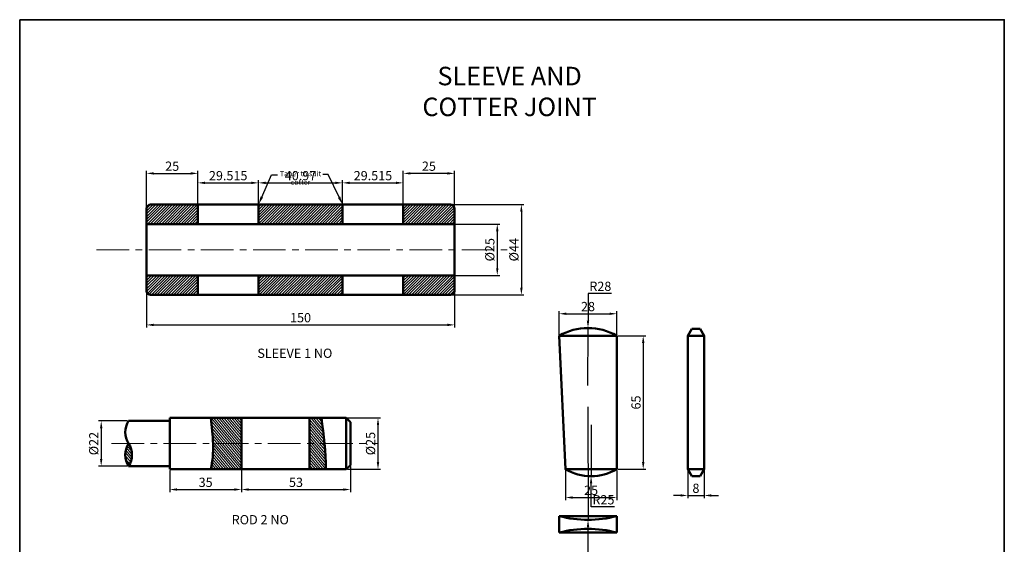
# Model space of a CAD drawing. Units: millimetres. Extents: x -431 to 49, y 153 to 670.
# Tile 2 of 2: x -431 to 49, y 415 to 670. Entities that reach past the tile are written whole.
import ezdxf
from ezdxf import colors
from ezdxf.entities.mleader import LeaderData, LeaderLine
from ezdxf.math import Vec2, Vec3

# ---------------------------------------------------------------- set-up
doc = ezdxf.new("R2010")
doc.units = ezdxf.units.MM
doc.header["$LTSCALE"] = 0.5
doc.linetypes.add('CENTER', pattern=[50.8, 31.75, -6.35, 6.35, -6.35])
for name, color, linetype, lineweight in [('M-CNTR', 1, 'CENTER', 18), ('M-DIMS', 2, 'Continuous', 25), ('M-HATC', 8, 'Continuous', 18), ('M-OUTL', 7, 'Continuous', 50), ('M-TEXT', 3, 'Continuous', 25), ('M-TTLB', 7, 'Continuous', 35)]:
    doc.layers.add(name, color=color, linetype=linetype, lineweight=lineweight)
doc.styles.get("Standard").update_dxf_attribs({"font": 'arial.ttf'})
doc.dimstyles.new('ISO-25', dxfattribs={"dimtxt": 4.5, "dimasz": 3.5, "dimexe": 1.25, "dimexo": 0.625, "dimtad": 1, "dimtoh": 1, "dimdec": 0, "dimtxsty": 'Standard', "dimcen": 2.5, "dimadec": 0, "dimazin": 0, "dimtfac": 1, "dimtdec": 0, "dimtmove": 0, "dimatfit": 3, "dimfxl": 1, "dimarcsym": 0})
pattern_1 = [(130, (-481.5719, 388.8533), (-0.7296573, -0.612255), [])]

# ---------------------------------------------------------------- blocks, each defined once
blk = doc.blocks.new('*D1')
at = {"layer": 'Defpoints', "color": 0, "transparency": 16777216}
for p in [(-343.88, 595.4), (-368.88, 570.74), (-343.88, 570.74)]:
    blk.add_point(p, dxfattribs=at)
at = {"layer": 'M-DIMS', "color": 0, "lineweight": -2, "transparency": 16777216}
for p, q in [((-368.88, 571.36), (-368.88, 596.65)), ((-365.38, 595.4), (-347.38, 595.4)), ((-343.88, 571.36), (-343.88, 596.65))]:
    blk.add_line(p, q, dxfattribs=at)
at = {"layer": 'M-DIMS', "color": 0, "transparency": 16777216}
for points in [[(-365.38, 595.98), (-365.38, 594.81), (-368.88, 595.4)], [(-347.38, 595.98), (-347.38, 594.81), (-343.88, 595.4)]]:
    blk.add_solid(points, dxfattribs=at)
at = {"layer": 'M-DIMS', "color": 0, "transparency": 16777216, "insert": (-356.38, 598.32), "char_height": 4.5, "attachment_point": 5}
blk.add_mtext('25', dxfattribs=at)
blk = doc.blocks.new('*D2')
at = {"layer": 'Defpoints', "color": 0, "transparency": 16777216}
for p in [(-243.88, 595.4), (-243.88, 570.74), (-218.88, 568.82)]:
    blk.add_point(p, dxfattribs=at)
at = {"layer": 'M-DIMS', "color": 0, "lineweight": -2, "transparency": 16777216}
for p, q in [((-243.88, 571.36), (-243.88, 596.65)), ((-222.38, 595.4), (-240.38, 595.4)), ((-218.88, 569.45), (-218.88, 596.65))]:
    blk.add_line(p, q, dxfattribs=at)
at = {"layer": 'M-DIMS', "color": 0, "transparency": 16777216}
for points in [[(-240.38, 595.98), (-240.38, 594.81), (-243.88, 595.4)], [(-222.38, 595.98), (-222.38, 594.81), (-218.88, 595.4)]]:
    blk.add_solid(points, dxfattribs=at)
at = {"layer": 'M-DIMS', "color": 0, "transparency": 16777216, "insert": (-231.38, 598.32), "char_height": 4.5, "attachment_point": 5}
blk.add_mtext('25', dxfattribs=at)
blk = doc.blocks.new('*D3')
at = {"layer": 'Defpoints', "color": 0, "transparency": 16777216}
for p in [(-368.88, 551.47), (-218.88, 551.47), (-218.88, 521.66)]:
    blk.add_point(p, dxfattribs=at)
at = {"layer": 'M-DIMS', "color": 0, "lineweight": -2, "transparency": 16777216}
for p, q in [((-368.88, 550.84), (-368.88, 520.41)), ((-218.88, 550.84), (-218.88, 520.41)), ((-365.38, 521.66), (-222.38, 521.66))]:
    blk.add_line(p, q, dxfattribs=at)
at = {"layer": 'M-DIMS', "color": 0, "transparency": 16777216}
for points in [[(-365.38, 522.24), (-365.38, 521.07), (-368.88, 521.66)], [(-222.38, 522.24), (-222.38, 521.07), (-218.88, 521.66)]]:
    blk.add_solid(points, dxfattribs=at)
at = {"layer": 'M-DIMS', "color": 0, "transparency": 16777216, "insert": (-293.88, 524.58), "char_height": 4.5, "attachment_point": 5}
blk.add_mtext('150', dxfattribs=at)
blk = doc.blocks.new('*D4')
at = {"layer": 'Defpoints', "color": 0, "transparency": 16777216}
for p in [(-228.43, 580.24), (-228.43, 536.24), (-186.36, 536.24)]:
    blk.add_point(p, dxfattribs=at)
at = {"layer": 'M-DIMS', "color": 0, "lineweight": -2, "transparency": 16777216}
for p, q in [((-227.8, 580.24), (-185.11, 580.24)), ((-186.36, 576.74), (-186.36, 539.74)), ((-227.8, 536.24), (-185.11, 536.24))]:
    blk.add_line(p, q, dxfattribs=at)
at = {"layer": 'M-DIMS', "color": 0, "transparency": 16777216}
for points in [[(-186.94, 576.74), (-185.77, 576.74), (-186.36, 580.24)], [(-186.94, 539.74), (-185.77, 539.74), (-186.36, 536.24)]]:
    blk.add_solid(points, dxfattribs=at)
at = {"layer": 'M-DIMS', "color": 0, "transparency": 16777216, "insert": (-189.41, 558.24), "char_height": 4.5, "attachment_point": 5, "rotation": 90}
blk.add_mtext('%%C44', dxfattribs=at)
blk = doc.blocks.new('*D5')
at = {"layer": 'Defpoints', "color": 0, "transparency": 16777216}
for p in [(-218.88, 570.74), (-218.88, 545.74), (-198.09, 545.74)]:
    blk.add_point(p, dxfattribs=at)
at = {"layer": 'M-DIMS', "color": 0, "lineweight": -2, "transparency": 16777216}
for p, q in [((-218.25, 570.74), (-196.84, 570.74)), ((-198.09, 567.24), (-198.09, 549.24)), ((-218.25, 545.74), (-196.84, 545.74))]:
    blk.add_line(p, q, dxfattribs=at)
at = {"layer": 'M-DIMS', "color": 0, "transparency": 16777216}
for points in [[(-198.68, 567.24), (-197.51, 567.24), (-198.09, 570.74)], [(-198.68, 549.24), (-197.51, 549.24), (-198.09, 545.74)]]:
    blk.add_solid(points, dxfattribs=at)
at = {"layer": 'M-DIMS', "color": 0, "transparency": 16777216, "insert": (-201.14, 558.24), "char_height": 4.5, "attachment_point": 5, "rotation": 90}
blk.add_mtext('%%C25', dxfattribs=at)
blk = doc.blocks.new('*D6')
at = {"layer": 'Defpoints', "color": 0, "transparency": 16777216}
for p in [(-139.92, 527.08), (-167.92, 516.39), (-139.92, 516.39)]:
    blk.add_point(p, dxfattribs=at)
at = {"layer": 'M-DIMS', "color": 0, "lineweight": -2, "transparency": 16777216}
for p, q in [((-167.92, 517.01), (-167.92, 528.33)), ((-139.92, 517.01), (-139.92, 528.33)), ((-164.42, 527.08), (-143.42, 527.08))]:
    blk.add_line(p, q, dxfattribs=at)
at = {"layer": 'M-DIMS', "color": 0, "transparency": 16777216}
for points in [[(-164.42, 527.66), (-164.42, 526.49), (-167.92, 527.08)], [(-143.42, 527.66), (-143.42, 526.49), (-139.92, 527.08)]]:
    blk.add_solid(points, dxfattribs=at)
at = {"layer": 'M-DIMS', "color": 0, "transparency": 16777216, "insert": (-153.92, 530), "char_height": 4.5, "attachment_point": 5}
blk.add_mtext('28', dxfattribs=at)
blk = doc.blocks.new('*D7')
at = {"layer": 'Defpoints', "color": 0, "transparency": 16777216}
for p in [(-164.92, 451.39), (-139.92, 451.39), (-139.92, 437.64)]:
    blk.add_point(p, dxfattribs=at)
at = {"layer": 'M-DIMS', "color": 0, "lineweight": -2, "transparency": 16777216}
for p, q in [((-164.92, 450.76), (-164.92, 436.39)), ((-139.92, 450.76), (-139.92, 436.39)), ((-161.42, 437.64), (-143.42, 437.64))]:
    blk.add_line(p, q, dxfattribs=at)
at = {"layer": 'M-DIMS', "color": 0, "transparency": 16777216}
for points in [[(-161.42, 438.22), (-161.42, 437.06), (-164.92, 437.64)], [(-143.42, 438.22), (-143.42, 437.06), (-139.92, 437.64)]]:
    blk.add_solid(points, dxfattribs=at)
at = {"layer": 'M-DIMS', "color": 0, "transparency": 16777216, "insert": (-152.42, 440.56), "char_height": 4.5, "attachment_point": 5}
blk.add_mtext('25', dxfattribs=at)
blk = doc.blocks.new('*D8')
at = {"layer": 'Defpoints', "color": 0, "transparency": 16777216}
for p in [(-139.92, 516.39), (-139.92, 451.39), (-127.04, 451.39)]:
    blk.add_point(p, dxfattribs=at)
at = {"layer": 'M-DIMS', "color": 0, "lineweight": -2, "transparency": 16777216}
for p, q in [((-139.29, 516.39), (-125.79, 516.39)), ((-127.04, 512.89), (-127.04, 454.89)), ((-139.29, 451.39), (-125.79, 451.39))]:
    blk.add_line(p, q, dxfattribs=at)
at = {"layer": 'M-DIMS', "color": 0, "transparency": 16777216}
for points in [[(-127.62, 512.89), (-126.45, 512.89), (-127.04, 516.39)], [(-127.62, 454.89), (-126.45, 454.89), (-127.04, 451.39)]]:
    blk.add_solid(points, dxfattribs=at)
at = {"layer": 'M-DIMS', "color": 0, "transparency": 16777216, "insert": (-129.96, 483.89), "char_height": 4.5, "attachment_point": 5, "rotation": 90}
blk.add_mtext('65', dxfattribs=at)
blk = doc.blocks.new('*D9')
at = {"layer": 'Defpoints', "color": 0, "transparency": 16777216}
for p in [(-105.35, 451.39), (-97.35, 451.39), (-97.35, 438.65)]:
    blk.add_point(p, dxfattribs=at)
at = {"layer": 'M-DIMS', "color": 0, "lineweight": -2, "transparency": 16777216}
for p, q in [((-105.35, 450.76), (-105.35, 437.4)), ((-97.35, 450.76), (-97.35, 437.4)), ((-108.85, 438.65), (-112.35, 438.65)), ((-105.35, 438.65), (-97.35, 438.65)), ((-93.85, 438.65), (-90.35, 438.65))]:
    blk.add_line(p, q, dxfattribs=at)
at = {"layer": 'M-DIMS', "color": 0, "transparency": 16777216}
for points in [[(-108.85, 439.23), (-108.85, 438.07), (-105.35, 438.65)], [(-93.85, 439.23), (-93.85, 438.07), (-97.35, 438.65)]]:
    blk.add_solid(points, dxfattribs=at)
at = {"layer": 'M-DIMS', "color": 0, "transparency": 16777216, "insert": (-101.35, 441.57), "char_height": 4.5, "attachment_point": 5}
blk.add_mtext('8', dxfattribs=at)
blk = doc.blocks.new('*D10')
at = {"layer": 'Defpoints', "color": 0, "transparency": 16777216}
for p in [(-271.6, 476.39), (-271.6, 451.39), (-256.17, 451.39)]:
    blk.add_point(p, dxfattribs=at)
at = {"layer": 'M-DIMS', "color": 0, "lineweight": -2, "transparency": 16777216}
for p, q in [((-270.98, 476.39), (-254.92, 476.39)), ((-256.17, 472.89), (-256.17, 454.89)), ((-270.98, 451.39), (-254.92, 451.39))]:
    blk.add_line(p, q, dxfattribs=at)
at = {"layer": 'M-DIMS', "color": 0, "transparency": 16777216}
for points in [[(-256.75, 472.89), (-255.58, 472.89), (-256.17, 476.39)], [(-256.75, 454.89), (-255.58, 454.89), (-256.17, 451.39)]]:
    blk.add_solid(points, dxfattribs=at)
at = {"layer": 'M-DIMS', "color": 0, "transparency": 16777216, "insert": (-259.21, 463.89), "char_height": 4.5, "attachment_point": 5, "rotation": 90}
blk.add_mtext('%%C25', dxfattribs=at)
blk = doc.blocks.new('*D11')
at = {"layer": 'Defpoints', "color": 0, "transparency": 16777216}
for p in [(-357.6, 451.39), (-322.6, 451.39), (-322.6, 441.53)]:
    blk.add_point(p, dxfattribs=at)
at = {"layer": 'M-DIMS', "color": 0, "lineweight": -2, "transparency": 16777216}
for p, q in [((-357.6, 450.77), (-357.6, 440.28)), ((-322.6, 450.77), (-322.6, 440.28)), ((-354.1, 441.53), (-326.1, 441.53))]:
    blk.add_line(p, q, dxfattribs=at)
at = {"layer": 'M-DIMS', "color": 0, "transparency": 16777216}
for points in [[(-354.1, 442.11), (-354.1, 440.95), (-357.6, 441.53)], [(-326.1, 442.11), (-326.1, 440.95), (-322.6, 441.53)]]:
    blk.add_solid(points, dxfattribs=at)
at = {"layer": 'M-DIMS', "color": 0, "transparency": 16777216, "insert": (-340.1, 444.45), "char_height": 4.5, "attachment_point": 5}
blk.add_mtext('35', dxfattribs=at)
blk = doc.blocks.new('*D12')
at = {"layer": 'Defpoints', "color": 0, "transparency": 16777216}
for p in [(-322.6, 451.39), (-269.6, 453.39), (-269.6, 441.53)]:
    blk.add_point(p, dxfattribs=at)
at = {"layer": 'M-DIMS', "color": 0, "lineweight": -2, "transparency": 16777216}
for p, q in [((-322.6, 450.77), (-322.6, 440.28)), ((-269.6, 452.77), (-269.6, 440.28)), ((-319.1, 441.53), (-273.1, 441.53))]:
    blk.add_line(p, q, dxfattribs=at)
at = {"layer": 'M-DIMS', "color": 0, "transparency": 16777216}
for points in [[(-319.1, 442.11), (-319.1, 440.95), (-322.6, 441.53)], [(-273.1, 442.11), (-273.1, 440.95), (-269.6, 441.53)]]:
    blk.add_solid(points, dxfattribs=at)
at = {"layer": 'M-DIMS', "color": 0, "transparency": 16777216, "insert": (-296.1, 444.45), "char_height": 4.5, "attachment_point": 5}
blk.add_mtext('53', dxfattribs=at)
blk = doc.blocks.new('*D13')
at = {"layer": 'Defpoints', "color": 0, "transparency": 16777216}
for p in [(-377.6, 474.89), (-390.94, 452.89), (-377.6, 452.89)]:
    blk.add_point(p, dxfattribs=at)
at = {"layer": 'M-DIMS', "color": 0, "lineweight": -2, "transparency": 16777216}
for p, q in [((-378.23, 474.89), (-392.19, 474.89)), ((-390.94, 471.39), (-390.94, 456.39)), ((-378.23, 452.89), (-392.19, 452.89))]:
    blk.add_line(p, q, dxfattribs=at)
at = {"layer": 'M-DIMS', "color": 0, "transparency": 16777216}
for points in [[(-391.52, 471.39), (-390.36, 471.39), (-390.94, 474.89)], [(-391.52, 456.39), (-390.36, 456.39), (-390.94, 452.89)]]:
    blk.add_solid(points, dxfattribs=at)
at = {"layer": 'M-DIMS', "color": 0, "transparency": 16777216, "insert": (-393.99, 463.89), "char_height": 4.5, "attachment_point": 5, "rotation": 90}
blk.add_mtext('%%C22', dxfattribs=at)
blk = doc.blocks.new('COTTER-FRONT')
blk.add_lwpolyline([(28, 65), (28, 0), (3, 0), (0, 65)], close=True)
blk.add_arc((14, 40.75), 28, 60, 120)
blk = doc.blocks.new('COTTER-TOP')
for p, q in [((28, 8), (0, 8)), ((0, 8), (0, 0)), ((28, 0), (28, 8)), ((0, 0), (28, 0))]:
    blk.add_line(p, q)
for centre, start, end in [((14, 61.19), 255.2533, 284.7467), ((14, -53.19), 75.2533, 104.7467)]:
    blk.add_arc(centre, 55, start, end)
blk = doc.blocks.new('*D29')
at = {"layer": 'Defpoints', "color": 0, "ltscale": 0.5, "transparency": 16777216}
for p in [(-314.36, 590.79), (-343.88, 580.24), (-314.36, 580.24)]:
    blk.add_point(p, dxfattribs=at)
at = {"layer": 'M-DIMS', "color": 0, "lineweight": -2, "ltscale": 0.5, "transparency": 16777216}
for p, q in [((-343.88, 580.86), (-343.88, 592.04)), ((-340.38, 590.79), (-317.86, 590.79)), ((-314.36, 580.86), (-314.36, 592.04))]:
    blk.add_line(p, q, dxfattribs=at)
at = {"layer": 'M-DIMS', "color": 0, "ltscale": 0.5, "transparency": 16777216}
for points in [[(-340.38, 591.37), (-340.38, 590.2), (-343.88, 590.79)], [(-317.86, 591.37), (-317.86, 590.2), (-314.36, 590.79)]]:
    blk.add_solid(points, dxfattribs=at)
at = {"layer": 'M-DIMS', "color": 0, "ltscale": 0.5, "transparency": 16777216, "insert": (-329.12, 593.71), "char_height": 4.5, "attachment_point": 5}
blk.add_mtext('29.515', dxfattribs=at)
blk = doc.blocks.new('*D30')
at = {"layer": 'Defpoints', "color": 0, "ltscale": 0.5, "transparency": 16777216}
for p in [(-273.39, 590.79), (-314.36, 580.24), (-273.39, 580.24)]:
    blk.add_point(p, dxfattribs=at)
at = {"layer": 'M-DIMS', "color": 0, "lineweight": -2, "ltscale": 0.5, "transparency": 16777216}
for p, q in [((-314.36, 580.86), (-314.36, 592.04)), ((-310.86, 590.79), (-276.89, 590.79)), ((-273.39, 580.86), (-273.39, 592.04))]:
    blk.add_line(p, q, dxfattribs=at)
at = {"layer": 'M-DIMS', "color": 0, "ltscale": 0.5, "transparency": 16777216}
for points in [[(-310.86, 591.37), (-310.86, 590.2), (-314.36, 590.79)], [(-276.89, 591.37), (-276.89, 590.2), (-273.39, 590.79)]]:
    blk.add_solid(points, dxfattribs=at)
at = {"layer": 'M-DIMS', "color": 0, "ltscale": 0.5, "transparency": 16777216, "insert": (-293.88, 593.71), "char_height": 4.5, "attachment_point": 5}
blk.add_mtext('40.97', dxfattribs=at)
blk = doc.blocks.new('*D31')
at = {"layer": 'Defpoints', "color": 0, "ltscale": 0.5, "transparency": 16777216}
for p in [(-243.88, 590.79), (-273.39, 580.24), (-243.88, 580.24)]:
    blk.add_point(p, dxfattribs=at)
at = {"layer": 'M-DIMS', "color": 0, "lineweight": -2, "ltscale": 0.5, "transparency": 16777216}
for p, q in [((-273.39, 580.86), (-273.39, 592.04)), ((-269.89, 590.79), (-247.38, 590.79)), ((-243.88, 580.86), (-243.88, 592.04))]:
    blk.add_line(p, q, dxfattribs=at)
at = {"layer": 'M-DIMS', "color": 0, "ltscale": 0.5, "transparency": 16777216}
for points in [[(-269.89, 591.37), (-269.89, 590.2), (-273.39, 590.79)], [(-247.38, 591.37), (-247.38, 590.2), (-243.88, 590.79)]]:
    blk.add_solid(points, dxfattribs=at)
at = {"layer": 'M-DIMS', "color": 0, "ltscale": 0.5, "transparency": 16777216, "insert": (-258.63, 593.71), "char_height": 4.5, "attachment_point": 5}
blk.add_mtext('29.515', dxfattribs=at)
blk = doc.blocks.new('*D32')
at = {"layer": 'Defpoints', "color": 0, "ltscale": 0.5, "transparency": 16777216}
for p in [(-153.91, 520.14), (-153.92, 492.14)]:
    blk.add_point(p, dxfattribs=at)
at = {"layer": 'M-DIMS', "color": 0, "lineweight": -2, "ltscale": 0.5, "transparency": 16777216}
for p, q in [((-142.53, 536.94), (-153.91, 536.94)), ((-153.91, 536.94), (-153.91, 523.64)), ((-153.92, 492.14), (-153.91, 520.14))]:
    blk.add_line(p, q, dxfattribs=at)
at = {"layer": 'M-DIMS', "color": 0, "ltscale": 0.5, "transparency": 16777216}
blk.add_solid([(-154.5, 523.64), (-153.33, 523.64), (-153.91, 520.14)], dxfattribs=at)
at = {"layer": 'M-DIMS', "color": 0, "ltscale": 0.5, "transparency": 16777216, "insert": (-147.91, 539.86), "char_height": 4.5, "attachment_point": 5}
blk.add_mtext('R28', dxfattribs=at)
blk = doc.blocks.new('*D33')
at = {"layer": 'Defpoints', "color": 0, "ltscale": 0.5, "transparency": 16777216}
for p in [(-152.42, 473.04), (-152.41, 448.04)]:
    blk.add_point(p, dxfattribs=at)
at = {"layer": 'M-DIMS', "color": 0, "lineweight": -2, "ltscale": 0.5, "transparency": 16777216}
for p, q in [((-152.42, 473.04), (-152.41, 448.04)), ((-152.41, 433.04), (-152.41, 444.54)), ((-141, 433.04), (-152.41, 433.04))]:
    blk.add_line(p, q, dxfattribs=at)
at = {"layer": 'M-DIMS', "color": 0, "ltscale": 0.5, "transparency": 16777216}
blk.add_solid([(-151.83, 444.54), (-153, 444.54), (-152.41, 448.04)], dxfattribs=at)
at = {"layer": 'M-DIMS', "color": 0, "ltscale": 0.5, "transparency": 16777216, "insert": (-146.4, 435.96), "char_height": 4.5, "attachment_point": 5}
blk.add_mtext('R25', dxfattribs=at)
blk = doc.blocks.new('*D34')
at = {"layer": 'Defpoints', "color": 0, "ltscale": 0.5, "transparency": 16777216}
for p in [(-153.92, 481.78), (-153.91, 426.78)]:
    blk.add_point(p, dxfattribs=at)
at = {"layer": 'M-DIMS', "color": 0, "lineweight": -2, "ltscale": 0.5, "transparency": 16777216}
for p, q in [((-153.92, 481.78), (-153.91, 426.78)), ((-153.91, 393.78), (-153.91, 423.28)), ((-132.76, 393.78), (-153.91, 393.78))]:
    blk.add_line(p, q, dxfattribs=at)
at = {"layer": 'M-DIMS', "color": 0, "ltscale": 0.5, "transparency": 16777216}
blk.add_solid([(-153.33, 423.28), (-154.5, 423.28), (-153.91, 426.78)], dxfattribs=at)
at = {"layer": 'M-DIMS', "color": 0, "ltscale": 0.5, "transparency": 16777216, "insert": (-143.02, 396.71), "char_height": 4.5, "attachment_point": 5}
blk.add_mtext('2X R55', dxfattribs=at)

msp = doc.modelspace()

# ---------------------------------------------------------------- hatches: boundary and pattern name
at = {"layer": 'M-HATC'}
h = msp.add_hatch(dxfattribs=at)
h.set_pattern_fill('ANSI31', color=256, scale=0.3)
h.set_pattern_definition([(45, (-481.5719, 388.8533), (-0.6735192, 0.6735192), [])])
h.paths.add_polyline_path([(-366.8758, 580.2379, 0.41421356), (-368.8758, 578.2379), (-368.8758, 570.7379), (-343.8758, 570.7379), (-343.8758, 580.2379)])
h.paths.add_polyline_path([(-314.3604, 580.2379), (-314.3604, 570.7379), (-273.3912, 570.7379), (-273.3912, 580.2379)])
h.paths.add_polyline_path([(-243.8758, 580.2379), (-243.8758, 570.7379), (-218.8758, 570.7379), (-218.8758, 578.2379, 0.41421356), (-220.8758, 580.2379)])
h.paths.add_polyline_path([(-243.8758, 545.7379), (-243.8758, 536.2379), (-220.8758, 536.2379, 0.41421356), (-218.8758, 538.2379), (-218.8758, 545.7379)])
h.paths.add_polyline_path([(-314.3604, 545.7379), (-314.3604, 536.2379), (-273.3912, 536.2379), (-273.3912, 545.7379)])
h.paths.add_polyline_path([(-368.8758, 545.7379), (-368.8758, 538.2379, 0.41421356), (-366.8758, 536.2379), (-343.8758, 536.2379), (-343.8758, 545.7379)])
h = msp.add_hatch(dxfattribs=at)
h.set_pattern_fill('ANSI31', color=256, scale=0.3, angle=85)
h.set_pattern_definition(pattern_1)
edge = h.paths.add_edge_path()
edge.add_line((-322.6016, 476.393), (-337.6381, 476.393))
edge.add_spline(control_points=[(-337.6381, 476.393), (-337.1447, 472.2053), (-336.6513, 468.0177), (-336.5163, 463.893)], knot_values=[0, 0, 0, 0, 12.30275825, 12.30275825, 12.30275825, 12.30275825], degree=3, periodic=0)
edge.add_line((-336.5163, 463.893), (-322.6016, 463.893))
edge.add_line((-322.6016, 463.893), (-322.6016, 476.393))
edge = h.paths.add_edge_path()
edge.add_line((-322.6016, 463.893), (-336.5163, 463.893))
edge.add_spline(control_points=[(-336.5163, 463.893), (-336.3771, 459.6361), (-336.6196, 455.4464), (-337.6381, 451.393)], knot_values=[12.30275825, 12.30275825, 12.30275825, 12.30275825, 25, 25, 25, 25], degree=3, periodic=0)
edge.add_line((-337.6381, 451.393), (-322.6016, 451.393))
edge.add_line((-322.6016, 451.393), (-322.6016, 463.893))
edge = h.paths.add_edge_path()
edge.add_spline(control_points=[(-282.2402, 463.893), (-282.636, 468.063), (-283.1464, 472.228), (-283.6569, 476.393)], knot_values=[0, 0, 0, 0, 12.56066367, 12.56066367, 12.56066367, 12.56066367], degree=3, periodic=0)
edge.add_line((-283.6569, 476.393), (-289.5247, 476.393))
edge.add_line((-289.5247, 476.393), (-289.5247, 463.893))
edge.add_line((-289.5247, 463.893), (-282.2402, 463.893))
edge = h.paths.add_edge_path()
edge.add_spline(control_points=[(-281.5119, 451.393), (-281.5646, 455.5678), (-281.8454, 459.7329), (-282.2402, 463.893)], knot_values=[12.56066367, 12.56066367, 12.56066367, 12.56066367, 25.09185019, 25.09185019, 25.09185019, 25.09185019], degree=3, periodic=0)
edge.add_line((-282.2402, 463.893), (-289.5247, 463.893))
edge.add_line((-289.5247, 463.893), (-289.5247, 451.393))
edge.add_line((-289.5247, 451.393), (-281.5119, 451.393))
h = msp.add_hatch(dxfattribs=at)
h.set_pattern_fill('ANSI31', color=256, scale=0.3, angle=85)
h.set_pattern_definition(pattern_1)
h.paths.add_polyline_path([(-377.6016, 463.893, 0.29970063), (-377.6016, 452.893, 0.29970063)])

# ---------------------------------------------------------------- linework, layer by layer
at = {"layer": 'M-CNTR'}
for p, q in [((-393.2224, 558.2379), (-192.0844, 558.2379)), ((-385.9533, 463.893), (-256.3955, 463.893))]:
    msp.add_line(p, q, dxfattribs=at)
at = {"layer": 'M-OUTL'}
for p, q in [((-220.8758, 580.2379), (-366.8758, 580.2379)), ((-343.8758, 580.2379), (-343.8758, 570.7379)), ((-314.3604, 580.2379), (-314.3604, 570.7379)), ((-271.3912, 580.2379), (-273.3912, 580.2379)), ((-273.3912, 580.2379), (-273.3912, 570.7379)), ((-243.8758, 570.7379), (-243.8758, 580.2379)), ((-368.8758, 578.2379), (-368.8758, 538.2379)), ((-218.8758, 538.2379), (-218.8758, 578.2379)), ((-368.8758, 570.7379), (-218.8758, 570.7379)), ((-368.8758, 545.7379), (-218.8758, 545.7379)), ((-343.8758, 545.7379), (-343.8758, 536.2379)), ((-314.3604, 545.7379), (-314.3604, 536.2379)), ((-273.3912, 545.7379), (-273.3912, 536.2379)), ((-243.8758, 536.2379), (-243.8758, 545.7379)), ((-366.8758, 536.2379), (-220.8758, 536.2379)), ((-103.3526, 519.737), (-105.3526, 516.3876)), ((-103.3526, 519.737), (-99.3526, 519.737)), ((-99.3526, 519.737), (-97.3526, 516.3876)), ((-105.3526, 516.3876), (-105.3526, 451.3876)), ((-97.3526, 516.3876), (-105.3526, 516.3876)), ((-97.3526, 451.3876), (-97.3526, 516.3876)), ((-357.6016, 474.893), (-377.6016, 474.893)), ((-357.6016, 476.393), (-271.6016, 476.393)), ((-357.6016, 451.393), (-357.6016, 476.393)), ((-322.6016, 451.393), (-322.6016, 476.393)), ((-289.5247, 476.393), (-289.5247, 451.393)), ((-271.6016, 476.393), (-269.6016, 474.393)), ((-271.6016, 476.393), (-271.6016, 451.393)), ((-269.6016, 474.393), (-269.6016, 453.393)), ((-377.6016, 452.893), (-357.6016, 452.893)), ((-271.6016, 451.393), (-357.6016, 451.393)), ((-271.6016, 451.393), (-269.6016, 453.393)), ((-105.3526, 451.3876), (-97.3526, 451.3876)), ((-103.3526, 448.0382), (-105.3526, 451.3876)), ((-99.3526, 448.0382), (-97.3526, 451.3876)), ((-103.3526, 448.0382), (-99.3526, 448.0382))]:
    msp.add_line(p, q, dxfattribs=at)
for centre, radius, start, end in [((-366.8758, 578.2379), 2, 90, 180), ((-220.8758, 578.2379), 2, 0, 90), ((-366.8758, 538.2379), 2, 180, 270), ((-220.8758, 538.2379), 2, 270, 0), ((-369.25, 469.393), 10, 146.632987, 213.367013), ((-369.25, 458.393), 10, 146.632987, 213.367013), ((-385.9533, 458.393), 10, 326.632987, 33.367013), ((-152.4154, 473.0382), 25, 240, 300)]:
    msp.add_arc(centre, radius, start, end, dxfattribs=at)
for points in [[(-337.6381, 476.393), (-336.6354, 467.8834), (-335.6328, 459.3738), (-337.6381, 451.393)], [(-283.6569, 476.393), (-282.6372, 468.0727), (-281.6175, 459.7525), (-281.5119, 451.393)]]:
    msp.add_open_spline(points, degree=3, dxfattribs=at)
at = {"layer": 'M-TTLB', "ltscale": 0.5}
msp.add_lwpolyline([(-430.6355, 670.1955), (48.7912, 670.1955), (48.7912, 152.7108), (-430.6355, 152.7108)], close=True, dxfattribs=at)

# ---------------------------------------------------------------- block references
at = {"layer": 'M-OUTL'}
for name, p in [('COTTER-FRONT', (-167.915, 451.388)), ('COTTER-TOP', (-167.915, 420.597))]:
    msp.add_blockref(name, p, dxfattribs=at)

# ---------------------------------------------------------------- texts
at = {"layer": 'M-TEXT', "attachment_point": 1}
for s, width, insert, char_height in [('\\pxqc;SLEEVE AND COTTER JOINT', 108.244216, (-246.2093, 647.2727), 9), ('\\pxqc;Taper to suit\\Pcotter', 20.904088, (-304.3393, 596.5411), 2.5), ('\\pxqc;SLEEVE 1 NO', 77.714637, (-335.509, 510.1081), 4.5), ('\\pxqc;ROD 2 NO', 77.714637, (-352.3477, 429.104), 4.5)]:
    msp.add_mtext_dynamic_manual_height_columns(s, width=width, gutter_width=12.5, heights=[0], dxfattribs=dict(at, insert=insert, char_height=char_height))

# ---------------------------------------------------------------- dimensions: what is measured, and where the dimension line sits
at = {"layer": 'M-DIMS'}
for base, p1, p2, picture, middle in [((-343.8758, 595.3958), (-368.8758, 570.7379), (-343.8758, 570.7379), '*D1', (-356.3758, 598.3183)), ((-243.8758, 595.3958), (-218.8758, 568.8234), (-243.8758, 570.7379), '*D2', (-231.3758, 598.3183)), ((-218.8758, 521.6556), (-368.8758, 551.4686), (-218.8758, 551.4686), '*D3', (-293.8758, 524.5781)), ((-139.9154, 527.0752), (-167.9154, 516.3876), (-139.9154, 516.3876), '*D6', (-153.9154, 529.9978)), ((-322.6016, 441.5308), (-357.6016, 451.393), (-322.6016, 451.393), '*D11', (-340.1016, 444.4549)), ((-269.6016, 441.5308), (-322.6016, 451.393), (-269.6016, 453.393), '*D12', (-296.1016, 444.4549)), ((-97.3526, 438.6493), (-105.3526, 451.3876), (-97.3526, 451.3876), '*D9', (-101.3526, 441.5719))]:
    dim = msp.add_linear_dim(base=base, p1=p1, p2=p2, dimstyle='ISO-25', override={"dimclrd": 0, "dimclre": 0, "dimclrt": 0}, dxfattribs=at)
    dim.commit()
    dim.dimension.update_dxf_attribs({"geometry": picture, "text_midpoint": middle})
at = {"layer": 'M-DIMS', "ltscale": 0.5}
for base, p1, p2, override, picture, middle in [((-314.3604, 590.7879), (-343.8758, 580.2379), (-314.3604, 580.2379), {"dimdec": 3, "dimlfac": 1, "dimrnd": 0, "dimzin": 0, "dimdsep": 46, "dimlunit": 2}, '*D29', (-329.1181, 593.7104)), ((-273.3912, 590.7879), (-314.3604, 580.2379), (-273.3912, 580.2379), {"dimdec": 2, "dimlfac": 1, "dimrnd": 0, "dimzin": 0, "dimdsep": 46, "dimlunit": 2}, '*D30', (-293.8758, 593.7104)), ((-243.8758, 590.7879), (-273.3912, 580.2379), (-243.8758, 580.2379), {"dimdec": 3, "dimlfac": 1, "dimrnd": 0, "dimzin": 0, "dimdsep": 46, "dimlunit": 2}, '*D31', (-258.6335, 593.7104))]:
    dim = msp.add_linear_dim(base=base, p1=p1, p2=p2, dimstyle='ISO-25', override=override, dxfattribs=at)
    dim.commit()
    dim.dimension.update_dxf_attribs({"geometry": picture, "text_midpoint": middle})
at = {"layer": 'M-DIMS'}
for base, p1, p2, picture, middle in [((-186.3566, 536.2379), (-228.4285, 580.2379), (-228.4285, 536.2379), '*D4', (-189.405, 558.2379)), ((-198.0943, 545.7379), (-218.8758, 570.7379), (-218.8758, 545.7379), '*D5', (-201.1427, 558.2379)), ((-390.9413, 452.893), (-377.6016, 474.893), (-377.6016, 452.893), '*D13', (-393.9897, 463.893)), ((-256.1657, 451.393), (-271.6016, 476.393), (-271.6016, 451.393), '*D10', (-259.2141, 463.893))]:
    dim = msp.add_linear_dim(base=base, p1=p1, p2=p2, angle=90, text='%%C<>', dimstyle='ISO-25', override={"dimclrd": 0, "dimclre": 0, "dimclrt": 0}, dxfattribs=at)
    dim.commit()
    dim.dimension.update_dxf_attribs({"geometry": picture, "text_midpoint": middle})
at = {"layer": 'M-DIMS', "ltscale": 0.5}
for center, mpoint, picture, middle in [((-153.9154, 492.1389), (-153.915, 520.1389), '*D32', (-147.9088, 536.9389)), ((-152.4154, 473.0382), (-152.415, 448.0382), '*D33', (-146.3965, 433.0382))]:
    dim = msp.add_radius_dim(center=center, mpoint=mpoint, dimstyle='ISO-25', override={"dimdec": 0, "dimlfac": 1, "dimrnd": 0, "dimzin": 0, "dimdsep": 46, "dimlunit": 2}, dxfattribs=at)
    dim.commit()
    dim.dimension.update_dxf_attribs({"geometry": picture, "text_midpoint": middle, "dimtype": 164})
at = {"layer": 'M-DIMS'}
dim = msp.add_linear_dim(base=(-127.0355, 451.3876), p1=(-139.9154, 516.3876), p2=(-139.9154, 451.3876), angle=90, dimstyle='ISO-25', override={"dimclrd": 0, "dimclre": 0, "dimclrt": 0}, dxfattribs=at)
dim.commit()
dim.dimension.update_dxf_attribs({"geometry": '*D8', "text_midpoint": (-129.9581, 483.8876)})
at = {"layer": 'M-DIMS', "ltscale": 0.5}
dim = msp.add_radius_dim(center=(-153.9154, 481.785), mpoint=(-153.915, 426.785), text='2X <>', dimstyle='ISO-25', override={"dimdec": 0, "dimlfac": 1, "dimrnd": 0, "dimzin": 0, "dimdsep": 46, "dimlunit": 2}, dxfattribs=at)
dim.commit()
dim.dimension.update_dxf_attribs({"geometry": '*D34', "text_midpoint": (-143.0236, 393.785), "dimtype": 164})
at = {"layer": 'M-DIMS'}
dim = msp.add_linear_dim(base=(-139.9154, 437.6387), p1=(-164.9154, 451.3876), p2=(-139.9154, 451.3876), dimstyle='ISO-25', override={"dimclrd": 0, "dimclre": 0, "dimclrt": 0}, dxfattribs=at)
dim.commit()
dim.dimension.update_dxf_attribs({"geometry": '*D7', "text_midpoint": (-152.4154, 437.6387), "dimtype": 160})

# ---------------------------------------------------------------- leaders
ml = msp.add_multileader_mtext('Standard', dxfattribs=at)
ml.set_content('', color=256)
ml.set_leader_properties()
ml.build(insert=Vec2(0, 0))
ctx = ml.context
ctx.base_point, ctx.plane_origin = Vec3(-305.1029, 594.6346), Vec3(-314.3604, 580.2379)
notes = []
notes.append((ctx, [(0, (1, 1, 0), (-308.0039, 594.6346), (1, 0), 2.901, [(0, [(-314.3604, 580.2379)], 0, [])])]))
ctx.mtext.insert, ctx.mtext.flow_direction = Vec3(-303.1029, 596.6346), 5
ml = msp.add_multileader_mtext('Standard', dxfattribs=at)
ml.set_content('', color=256)
ml.set_leader_properties()
ml.build(insert=Vec2(0, 0))
ctx = ml.context
ctx.base_point, ctx.plane_origin = Vec3(-287.0057, 594.7869), Vec3(-273.3912, 580.2379)
ctx.text_align_type = 2
notes.append((ctx, [(0, (1, 1, 0), (-280.4788, 594.7869), (-1, 0), 2.5269, [(0, [(-273.3912, 580.2379)], 0, [])])]))
ctx.mtext.insert, ctx.mtext.alignment, ctx.mtext.flow_direction = Vec3(-285.0057, 596.7869), 3, 5
for ctx, leaders in notes:
    for number, flags, end, landing, length, lines in leaders:
        leader = LeaderData()
        leader.index, (leader.has_last_leader_line, leader.has_dogleg_vector, leader.attachment_direction) = number, flags
        leader.last_leader_point, leader.dogleg_vector, leader.dogleg_length = Vec3(end), Vec3(landing), length
        for number, points, colour, breaks in lines:
            line = LeaderLine()
            line.index, line.vertices, line.color, line.breaks = number, Vec3.list(points), colors.encode_raw_color(colour), breaks
            leader.lines.append(line)
        ctx.leaders.append(leader)

doc.saveas('drawing.dxf')
